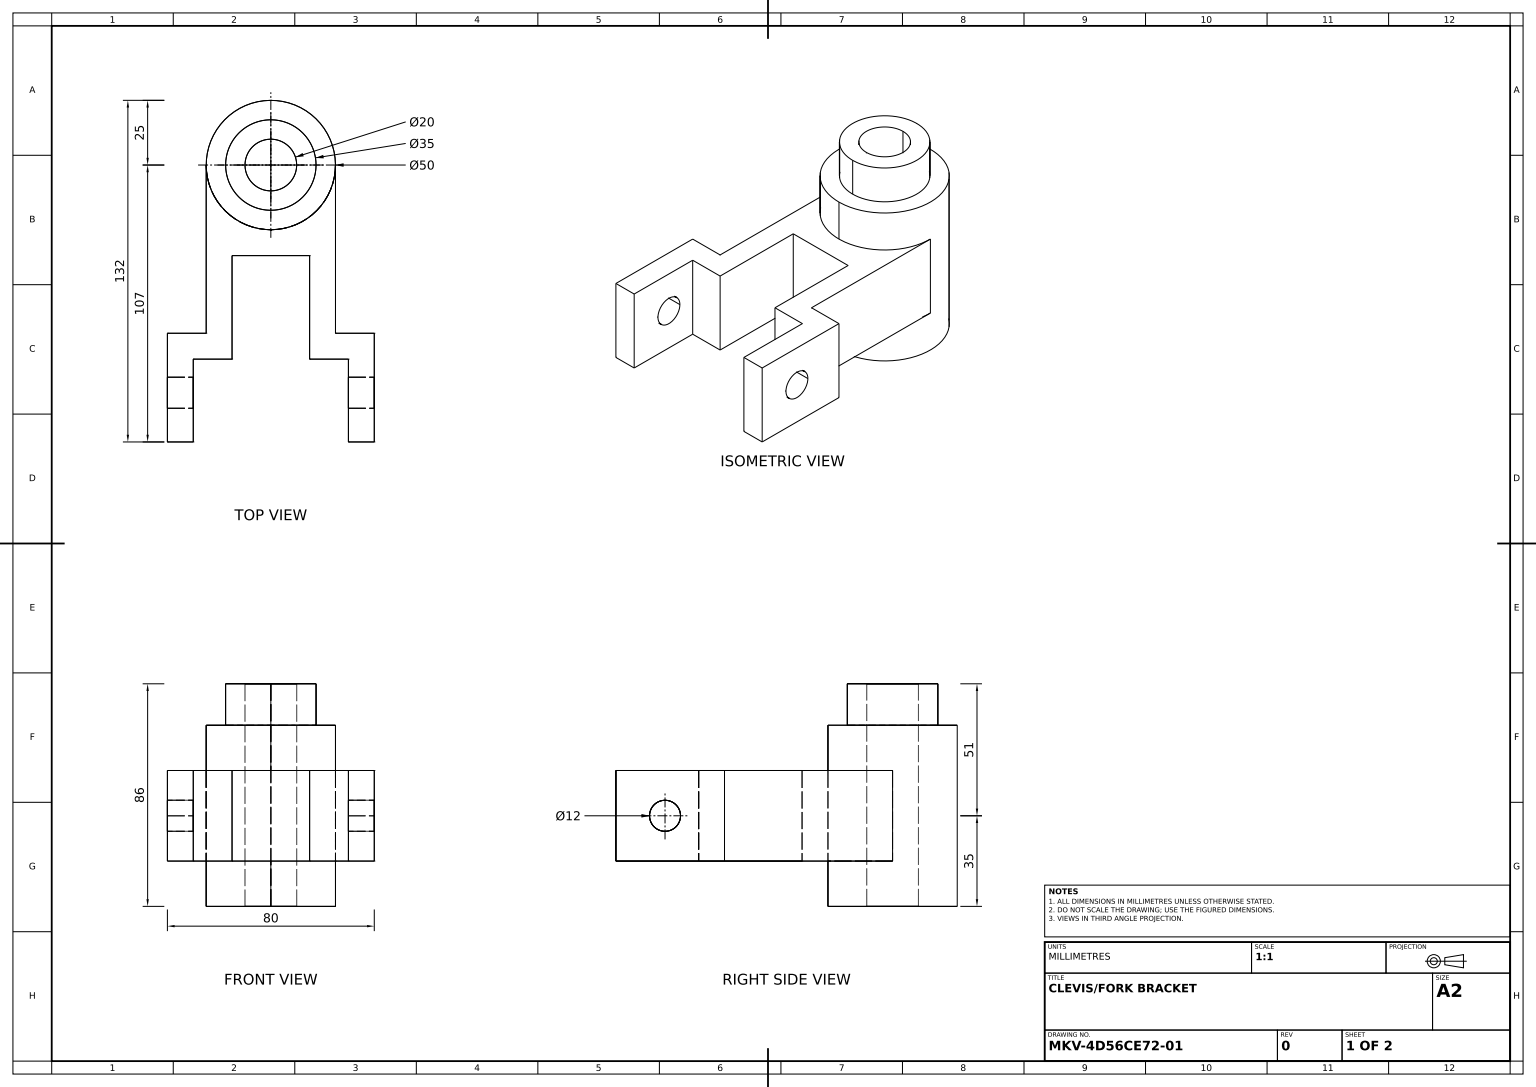
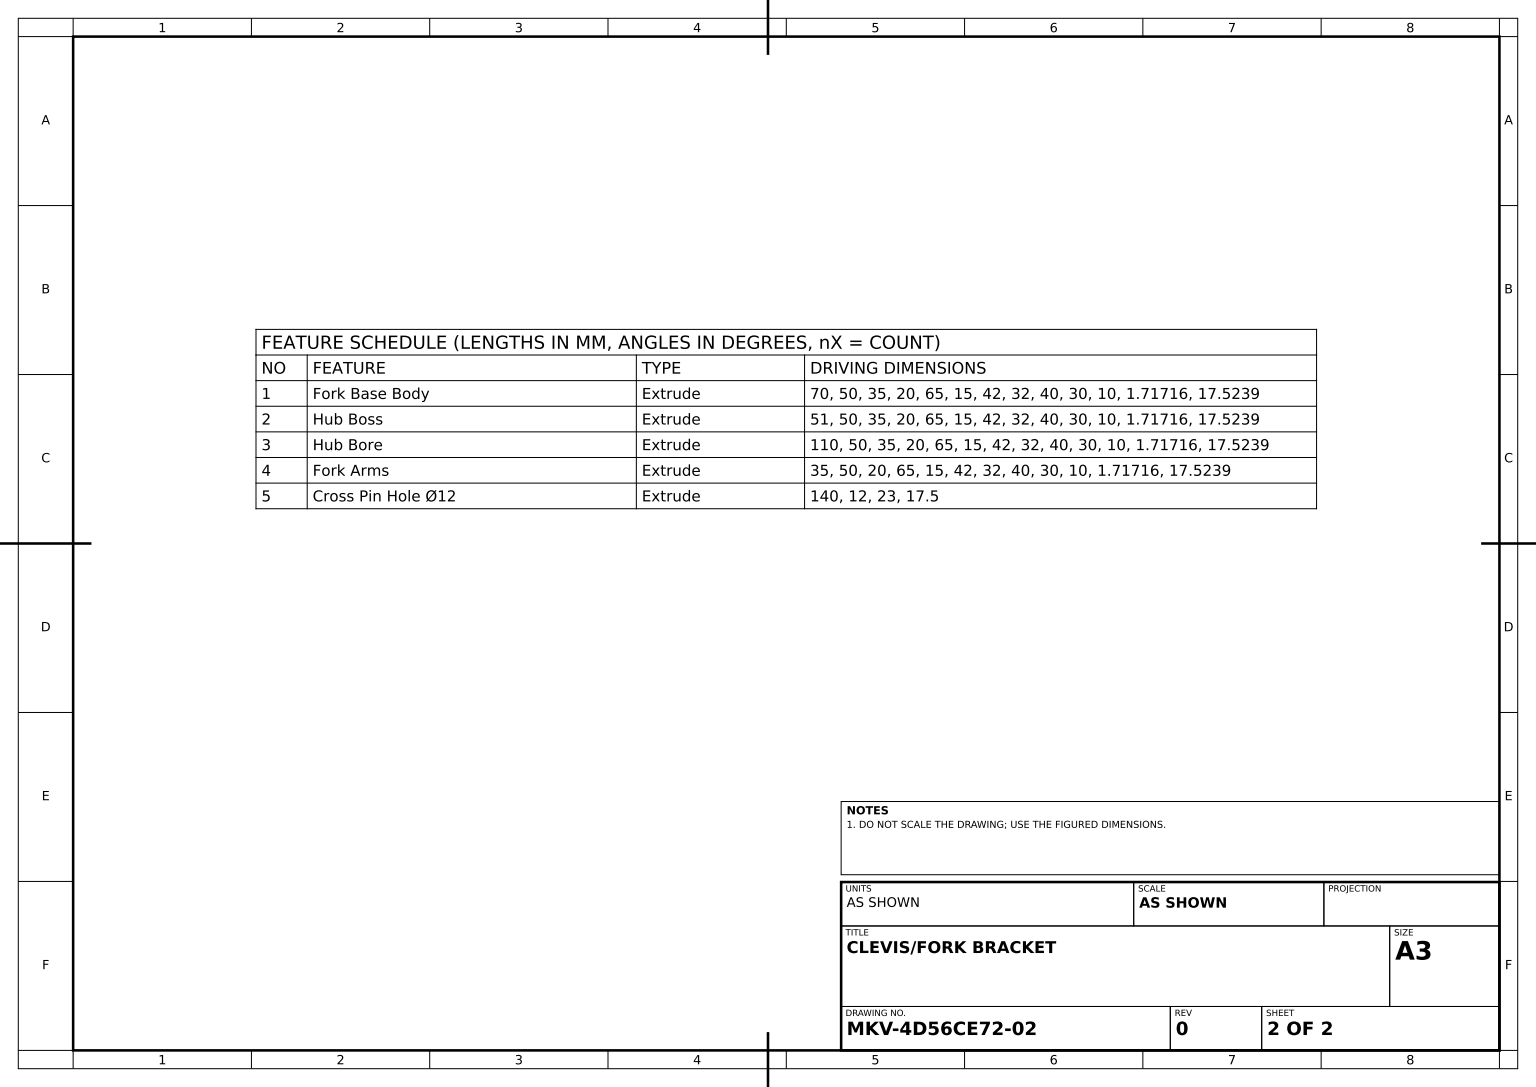
from build123d import *

# Parameters (mm, degrees)
FORK_PROFILE_SKETCH_R   = 25
FORK_BASE_BODY_DEPTH    = 35
SKETCH2_3_R             = 17.5
HUB_BOSS_DEPTH          = 51
HUB_BORE_DEPTH          = 55
FORK_ARMS_DEPTH         = 17.5
PIN_HOLE_SKETCH_R       = 6
CROSS_PIN_HOLE_12_DEPTH = 140


with BuildPart() as part:
    # Fork Profile Sketch → Fork Base Body (new, symmetric)
    with BuildSketch(Plane(origin=(0, 0, 0), x_dir=(1, 0, 0), z_dir=(0, 1, 0))):
        with Locations(Location((0, 0, 0), (0, 0, 270))):
            Circle(FORK_PROFILE_SKETCH_R)
    extrude(amount=FORK_BASE_BODY_DEPTH, both=True)

    # Sketch2_3 → Hub Boss (add)
    with BuildSketch(Plane(origin=(0, 0, 0), x_dir=(1, 0, 0), z_dir=(0, 1, 0))):
        with Locations(Location((0, 0, 0), (0, 0, 270))):
            Circle(SKETCH2_3_R)
    extrude(amount=HUB_BOSS_DEPTH)

    # Sketch2_4 → Hub Bore (cut, symmetric)
    with BuildSketch(Plane(origin=(0, 0, 0), x_dir=(1, 0, 0), z_dir=(0, 1, 0))):
        with BuildLine():
            Line((9.946400687, -1.033979392), (0, -1.717163069))
            Line((0, -1.717163069), (-9.946400687, -1.033979392))
            ThreePointArc((-9.946400687, -1.033979392), (0, -10), (9.946400687, -1.033979392))
        make_face()
        with BuildLine():
            Line((-9.946400687, -1.033979392), (0, -1.717163069))
            Line((0, -1.717163069), (9.946400687, -1.033979392))
            ThreePointArc((9.946400687, -1.033979392), (9.986591182, -0.517683849), (10, 0))
            ThreePointArc((10, 0), (-0.517683849, 9.986591182), (-9.946400687, -1.033979392))
        make_face()
        with BuildLine():
            Line((9.946400687, -1.033979392), (0, -1.717163069))
            Line((0, -1.717163069), (-9.946400687, -1.033979392))
            ThreePointArc((-9.946400687, -1.033979392), (0, -10), (9.946400687, -1.033979392))
        make_face()
        with BuildLine():
            Line((-9.946400687, -1.033979392), (0, -1.717163069))
            Line((0, -1.717163069), (9.946400687, -1.033979392))
            ThreePointArc((9.946400687, -1.033979392), (9.986591182, -0.517683849), (10, 0))
            ThreePointArc((10, 0), (-0.517683849, 9.986591182), (-9.946400687, -1.033979392))
        make_face()
    extrude(amount=HUB_BORE_DEPTH, both=True, mode=Mode.SUBTRACT)

    # Sketch2_5 → Fork Arms (add, symmetric)
    with BuildSketch(Plane(origin=(0, 0, 0), x_dir=(1, 0, 0), z_dir=(0, 1, 0))):
        with BuildLine():
            ThreePointArc((25, 0), (0, -25), (-25, 0))
            Line((-25, 0), (-25, -65))
            Line((-25, -65), (-40, -65))
            Line((-40, -65), (-40, -107))
            Line((-40, -107), (-30, -107))
            Line((-30, -107), (-30, -75))
            Line((-30, -75), (-15, -75))
            Line((-15, -75), (-15, -35))
            Line((-15, -35), (15, -35))
            Line((15, -35), (15, -52.523875455))
            Line((15, -52.523875455), (15, -75))
            Line((15, -75), (30, -75))
            Line((30, -75), (30, -107))
            Line((30, -107), (40, -107))
            Line((40, -107), (40, -65))
            Line((40, -65), (25, -65))
            Line((25, -65), (25, 0))
        make_face()
    extrude(amount=FORK_ARMS_DEPTH, both=True)

    # Pin Hole Sketch → Cross Pin Hole _12 (cut)
    with BuildSketch(Plane(origin=(40, 0, 0), x_dir=(0, 0, -1), z_dir=(1, 0, 0))):
        with Locations((-88, 0)):
            Circle(PIN_HOLE_SKETCH_R)
    extrude(amount=-CROSS_PIN_HOLE_12_DEPTH, mode=Mode.SUBTRACT)


solid = part.part
